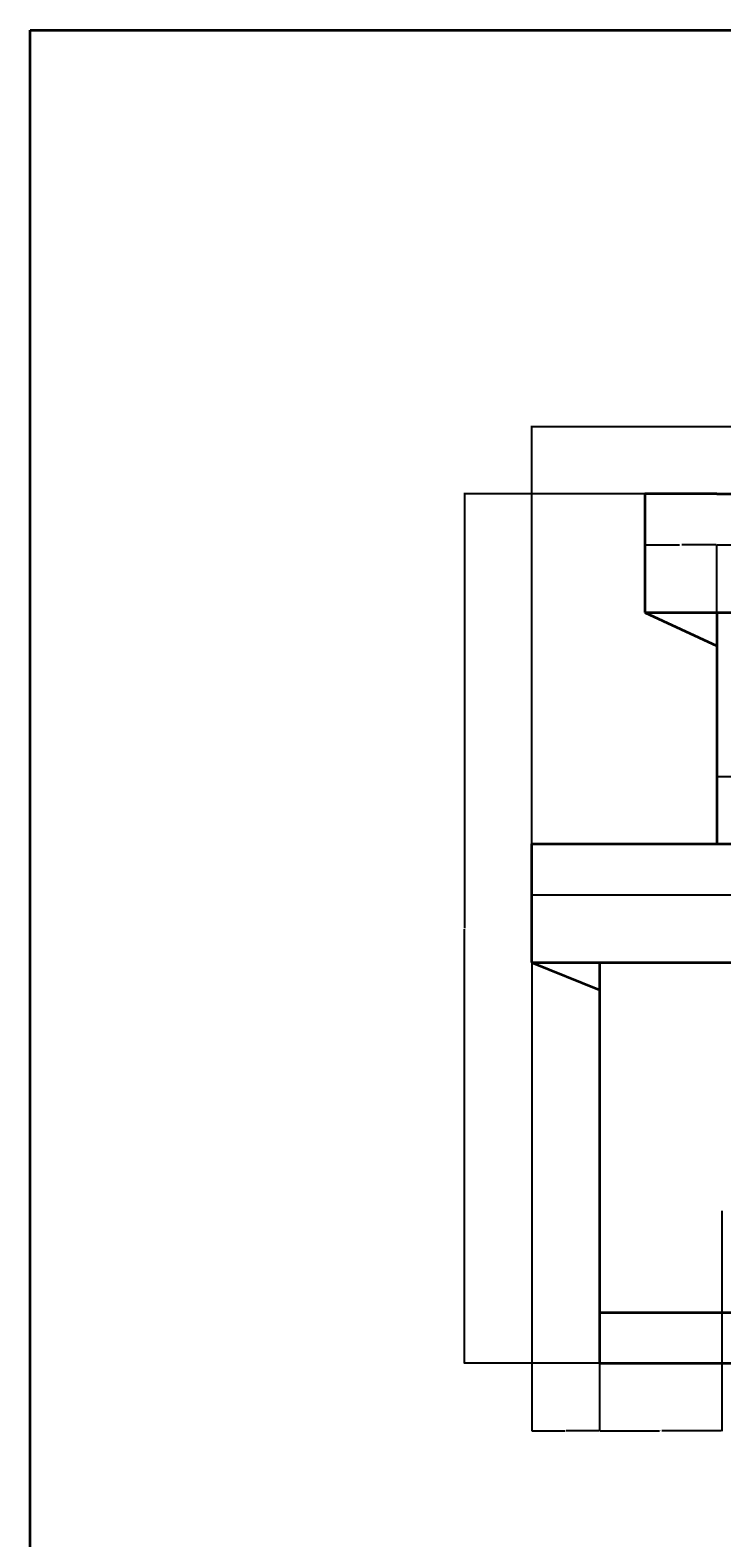
# Model space of a CAD drawing. Units: inches. Extents: x 2067 to 3463, y 1605 to 2723.
# Tile 6 of 10: x 2067 to 2312, y 2189 to 2723. Entities that reach past the tile are written whole.
import ezdxf

# ---------------------------------------------------------------- set-up
doc = ezdxf.new("R2010")
doc.units = ezdxf.units.IN
for name, color, linetype, lineweight in [('A-ANNO-DIMS', 2, 'Continuous', 18), ('A-ANNO-TTLB', 7, 'Continuous', 35), ('A-ELEV', 7, 'Continuous', 35)]:
    doc.layers.add(name, color=color, linetype=linetype, lineweight=lineweight)
doc.styles.get("Standard").update_dxf_attribs({"font": 'arial.ttf'})
doc.dimstyles.get("Standard").update_dxf_attribs({"dimtxt": 0.18, "dimasz": 0.18, "dimexe": 0.18, "dimexo": 0.0625, "dimgap": 0.09, "dimtad": 0, "dimtih": 1, "dimtoh": 1, "dimdec": 4, "dimzin": 0, "dimdsep": 46, "dimtxsty": 'Standard', "dimcen": 0.09, "dimadec": 0, "dimazin": 0, "dimtfac": 1, "dimtdec": 4, "dimtofl": 0, "dimtmove": 0, "dimatfit": 3, "dimfxl": 1, "dimtolj": 1, "dimtzin": 0, "dimarcsym": 0})

# ---------------------------------------------------------------- blocks, each defined once
blk = doc.blocks.new('*D69')
at = {"layer": 'A-ANNO-DIMS', "color": 0, "lineweight": -2, "transparency": 16777216}
for p, q in [((2244.95, 2434.43), (2244.95, 2582.45)), ((2245.13, 2582.27), (2475.3, 2582.27)), ((2706.27, 2582.27), (2476.1, 2582.27)), ((2706.45, 2558.43), (2706.45, 2582.45))]:
    blk.add_line(p, q, dxfattribs=at)
at = {"layer": 'A-ANNO-DIMS', "color": 0, "transparency": 16777216}
for points in [[(2245.13, 2582.3), (2245.13, 2582.24), (2244.95, 2582.27)], [(2706.27, 2582.3), (2706.27, 2582.24), (2706.45, 2582.27)]]:
    blk.add_solid(points, dxfattribs=at)
at = {"layer": 'Defpoints', "color": 0, "transparency": 16777216}
for p in [(2706.45, 2582.27), (2706.45, 2558.37), (2244.95, 2434.37)]:
    blk.add_point(p, dxfattribs=at)
at = {"layer": 'A-ANNO-DIMS', "color": 0, "transparency": 16777216, "insert": (2475.7, 2582.27), "char_height": 0.18, "attachment_point": 5}
blk.add_mtext('\\A1;461.5', dxfattribs=at)
blk = doc.blocks.new('*D70')
at = {"layer": 'A-ANNO-DIMS', "color": 0, "lineweight": -2, "transparency": 16777216}
for p, q in [((2284.87, 2558.37), (2220.87, 2558.37)), ((2221.05, 2558.19), (2221.05, 2404.55)), ((2221.05, 2250.55), (2221.05, 2404.18)), ((2268.89, 2250.37), (2220.87, 2250.37))]:
    blk.add_line(p, q, dxfattribs=at)
at = {"layer": 'A-ANNO-DIMS', "color": 0, "transparency": 16777216}
for points in [[(2221.02, 2558.19), (2221.08, 2558.19), (2221.05, 2558.37)], [(2221.02, 2250.55), (2221.08, 2250.55), (2221.05, 2250.37)]]:
    blk.add_solid(points, dxfattribs=at)
at = {"layer": 'Defpoints', "color": 0, "transparency": 16777216}
for p in [(2221.05, 2558.37), (2284.94, 2558.37), (2268.95, 2250.37)]:
    blk.add_point(p, dxfattribs=at)
at = {"layer": 'A-ANNO-DIMS', "color": 0, "transparency": 16777216, "insert": (2221.05, 2404.37), "char_height": 0.18, "attachment_point": 5}
blk.add_mtext('\\A1;308', dxfattribs=at)
blk = doc.blocks.new('*D77')
at = {"layer": 'A-ANNO-DIMS', "color": 0, "lineweight": -2, "transparency": 16777216}
for p, q in [((2284.94, 2516.43), (2284.94, 2540.45)), ((2285.12, 2540.27), (2297.31, 2540.27)), ((2310.27, 2540.27), (2298.07, 2540.27)), ((2310.45, 2516.43), (2310.45, 2540.45))]:
    blk.add_line(p, q, dxfattribs=at)
at = {"layer": 'A-ANNO-DIMS', "color": 0, "transparency": 16777216}
for points in [[(2285.12, 2540.3), (2285.12, 2540.24), (2284.94, 2540.27)], [(2310.27, 2540.3), (2310.27, 2540.24), (2310.45, 2540.27)]]:
    blk.add_solid(points, dxfattribs=at)
at = {"layer": 'Defpoints', "color": 0, "transparency": 16777216}
for p in [(2310.45, 2540.27), (2284.94, 2516.37), (2310.45, 2516.37)]:
    blk.add_point(p, dxfattribs=at)
at = {"layer": 'A-ANNO-DIMS', "color": 0, "transparency": 16777216, "insert": (2297.69, 2540.27), "char_height": 0.18, "attachment_point": 5}
blk.add_mtext('\\A1;25.51', dxfattribs=at)
blk = doc.blocks.new('*D78')
at = {"layer": 'A-ANNO-DIMS', "color": 0, "lineweight": -2, "transparency": 16777216}
for p, q in [((2310.45, 2516.43), (2310.45, 2540.45)), ((2310.63, 2540.27), (2382.81, 2540.27)), ((2455.77, 2540.27), (2383.58, 2540.27)), ((2455.95, 2516.43), (2455.95, 2540.45))]:
    blk.add_line(p, q, dxfattribs=at)
at = {"layer": 'A-ANNO-DIMS', "color": 0, "transparency": 16777216}
for points in [[(2310.63, 2540.3), (2310.63, 2540.24), (2310.45, 2540.27)], [(2455.77, 2540.3), (2455.77, 2540.24), (2455.95, 2540.27)]]:
    blk.add_solid(points, dxfattribs=at)
at = {"layer": 'Defpoints', "color": 0, "transparency": 16777216}
for p in [(2455.95, 2540.27), (2310.45, 2516.37), (2455.95, 2516.37)]:
    blk.add_point(p, dxfattribs=at)
at = {"layer": 'A-ANNO-DIMS', "color": 0, "transparency": 16777216, "insert": (2383.2, 2540.27), "char_height": 0.18, "attachment_point": 5}
blk.add_mtext('\\A1;145.5', dxfattribs=at)
blk = doc.blocks.new('*D81')
at = {"layer": 'A-ANNO-DIMS', "color": 0, "lineweight": -2, "transparency": 16777216}
for p, q in [((2310.45, 2434.43), (2310.45, 2458.45)), ((2310.63, 2458.27), (2322.63, 2458.27)), ((2335.38, 2458.27), (2323.38, 2458.27)), ((2335.56, 2434.43), (2335.56, 2458.45))]:
    blk.add_line(p, q, dxfattribs=at)
at = {"layer": 'A-ANNO-DIMS', "color": 0, "transparency": 16777216}
for points in [[(2310.63, 2458.3), (2310.63, 2458.24), (2310.45, 2458.27)], [(2335.38, 2458.3), (2335.38, 2458.24), (2335.56, 2458.27)]]:
    blk.add_solid(points, dxfattribs=at)
at = {"layer": 'Defpoints', "color": 0, "transparency": 16777216}
for p in [(2335.56, 2458.27), (2310.45, 2434.37), (2335.56, 2434.37)]:
    blk.add_point(p, dxfattribs=at)
at = {"layer": 'A-ANNO-DIMS', "color": 0, "transparency": 16777216, "insert": (2323, 2458.27), "char_height": 0.18, "attachment_point": 5}
blk.add_mtext('\\A1;25.11', dxfattribs=at)
blk = doc.blocks.new('*D90')
at = {"layer": 'A-ANNO-DIMS', "color": 0, "lineweight": -2, "transparency": 16777216}
for p, q in [((2244.95, 2392.3), (2244.95, 2226.29)), ((2268.95, 2250.3), (2268.95, 2226.29)), ((2245.13, 2226.47), (2256.73, 2226.47)), ((2268.77, 2226.47), (2257.17, 2226.47))]:
    blk.add_line(p, q, dxfattribs=at)
at = {"layer": 'A-ANNO-DIMS', "color": 0, "transparency": 16777216}
for points in [[(2245.13, 2226.5), (2245.13, 2226.44), (2244.95, 2226.47)], [(2268.77, 2226.5), (2268.77, 2226.44), (2268.95, 2226.47)]]:
    blk.add_solid(points, dxfattribs=at)
at = {"layer": 'Defpoints', "color": 0, "transparency": 16777216}
for p in [(2244.95, 2392.37), (2268.95, 2250.37), (2268.95, 2226.47)]:
    blk.add_point(p, dxfattribs=at)
at = {"layer": 'A-ANNO-DIMS', "color": 0, "transparency": 16777216, "insert": (2256.95, 2226.47), "char_height": 0.18, "attachment_point": 5}
blk.add_mtext('\\A1;24', dxfattribs=at)
blk = doc.blocks.new('*D91')
at = {"layer": 'A-ANNO-DIMS', "color": 0, "lineweight": -2, "transparency": 16777216}
for p, q in [((2312.26, 2304.3), (2312.26, 2226.29)), ((2268.95, 2250.3), (2268.95, 2226.29)), ((2269.13, 2226.47), (2290.22, 2226.47)), ((2312.08, 2226.47), (2290.98, 2226.47))]:
    blk.add_line(p, q, dxfattribs=at)
at = {"layer": 'A-ANNO-DIMS', "color": 0, "transparency": 16777216}
for points in [[(2269.13, 2226.5), (2269.13, 2226.44), (2268.95, 2226.47)], [(2312.08, 2226.5), (2312.08, 2226.44), (2312.26, 2226.47)]]:
    blk.add_solid(points, dxfattribs=at)
at = {"layer": 'Defpoints', "color": 0, "transparency": 16777216}
for p in [(2312.26, 2304.37), (2268.95, 2250.37), (2312.26, 2226.47)]:
    blk.add_point(p, dxfattribs=at)
at = {"layer": 'A-ANNO-DIMS', "color": 0, "transparency": 16777216, "insert": (2290.6, 2226.47), "char_height": 0.18, "attachment_point": 5}
blk.add_mtext('\\A1;43.31', dxfattribs=at)
blk = doc.blocks.new('*D99')
at = {"layer": 'A-ANNO-DIMS', "color": 0, "lineweight": -2, "transparency": 16777216}
for p, q in [((2244.95, 2392.43), (2244.95, 2416.45)), ((2245.13, 2416.27), (2364.7, 2416.27)), ((2485.06, 2416.27), (2365.49, 2416.27)), ((2485.24, 2392.43), (2485.24, 2416.45))]:
    blk.add_line(p, q, dxfattribs=at)
at = {"layer": 'A-ANNO-DIMS', "color": 0, "transparency": 16777216}
for points in [[(2245.13, 2416.3), (2245.13, 2416.24), (2244.95, 2416.27)], [(2485.06, 2416.3), (2485.06, 2416.24), (2485.24, 2416.27)]]:
    blk.add_solid(points, dxfattribs=at)
at = {"layer": 'Defpoints', "color": 0, "transparency": 16777216}
for p in [(2485.24, 2416.27), (2244.95, 2392.37), (2485.24, 2392.37)]:
    blk.add_point(p, dxfattribs=at)
at = {"layer": 'A-ANNO-DIMS', "color": 0, "transparency": 16777216, "insert": (2365.09, 2416.27), "char_height": 0.18, "attachment_point": 5}
blk.add_mtext('\\A1;240.3', dxfattribs=at)

msp = doc.modelspace()

# ---------------------------------------------------------------- linework, layer by layer
at = {"layer": 'A-ANNO-TTLB'}
msp.add_lwpolyline([(2067.2624, 2722.6321), (3463.3053, 2722.6321), (3463.3053, 1605.3918), (2067.2624, 1605.3918)], close=True, dxfattribs=at)
at = {"layer": 'A-ELEV'}
for p, q in [((2310.4477, 2558.3657), (2284.9353, 2558.3657)), ((2284.9353, 2558.3657), (2284.9353, 2516.3657)), ((2310.4477, 2558.3657), (2706.4477, 2558.3657)), ((2284.9353, 2516.3657), (2310.4477, 2516.3657)), ((2284.9353, 2516.3657), (2310.4477, 2504.4794)), ((2310.4477, 2516.3657), (2310.4477, 2434.3657)), ((2310.4477, 2516.3657), (2706.4477, 2516.3657)), ((2244.9477, 2434.3657), (2706.4477, 2434.3657)), ((2244.9477, 2392.3657), (2244.9477, 2434.3657)), ((2244.9477, 2392.3657), (2706.4477, 2392.3657)), ((2244.9477, 2392.3657), (2268.9477, 2382.6058)), ((2268.9477, 2392.3657), (2268.9477, 2250.3657)), ((2268.9477, 2268.3657), (2706.4477, 2268.3657)), ((2268.9477, 2250.3657), (2706.4477, 2250.3657))]:
    msp.add_line(p, q, dxfattribs=at)

# ---------------------------------------------------------------- dimensions: what is measured, and where the dimension line sits
at = {"layer": 'A-ANNO-DIMS'}
for base, p1, p2, override, picture, middle in [((2706.4477, 2582.2657), (2244.9477, 2434.3657), (2706.4477, 2558.3657), {"dimdec": 1, "dimlfac": 1, "dimrnd": 0, "dimzin": 0, "dimdsep": 46, "dimlunit": 2}, '*D69', (2475.6977, 2582.2657)), ((2310.4477, 2540.2657), (2284.9353, 2516.3657), (2310.4477, 2516.3657), {"dimdec": 2, "dimlfac": 1, "dimrnd": 0, "dimzin": 0, "dimdsep": 46, "dimlunit": 2}, '*D77', (2297.6915, 2540.2657)), ((2455.9477, 2540.2657), (2310.4477, 2516.3657), (2455.9477, 2516.3657), {"dimdec": 1, "dimlfac": 1, "dimrnd": 0, "dimzin": 0, "dimdsep": 46, "dimlunit": 2}, '*D78', (2383.1977, 2540.2657)), ((2335.5594, 2458.2657), (2310.4477, 2434.3657), (2335.5594, 2434.3657), {"dimdec": 2, "dimlfac": 1, "dimrnd": 0, "dimzin": 0, "dimdsep": 46, "dimlunit": 2}, '*D81', (2323.0035, 2458.2657)), ((2485.2361, 2416.2657), (2244.9477, 2392.3657), (2485.2361, 2392.3657), {"dimdec": 1, "dimlfac": 1, "dimrnd": 0, "dimzin": 0, "dimdsep": 46, "dimlunit": 2}, '*D99', (2365.0919, 2416.2657)), ((2268.9477, 2226.4657), (2244.9477, 2392.3657), (2268.9477, 2250.3657), {"dimdec": 0, "dimlfac": 1, "dimrnd": 0, "dimzin": 0, "dimdsep": 46, "dimlunit": 2}, '*D90', (2256.9477, 2226.4657)), ((2312.2608, 2226.4657), (2268.9477, 2250.3657), (2312.2608, 2304.3657), {"dimdec": 2, "dimlfac": 1, "dimrnd": 0, "dimzin": 0, "dimdsep": 46, "dimlunit": 2}, '*D91', (2290.6042, 2226.4657))]:
    dim = msp.add_linear_dim(base=base, p1=p1, p2=p2, dimstyle='Standard', override=override, dxfattribs=at)
    dim.commit()
    dim.dimension.update_dxf_attribs({"geometry": picture, "text_midpoint": middle})
dim = msp.add_linear_dim(base=(2221.0477, 2558.3657), p1=(2268.9477, 2250.3657), p2=(2284.9353, 2558.3657), angle=90, dimstyle='Standard', override={"dimdec": 0, "dimlfac": 1, "dimrnd": 0, "dimzin": 0, "dimdsep": 46, "dimlunit": 2}, dxfattribs=at)
dim.commit()
dim.dimension.update_dxf_attribs({"geometry": '*D70', "text_midpoint": (2221.0477, 2404.3657)})

doc.saveas('drawing.dxf')
